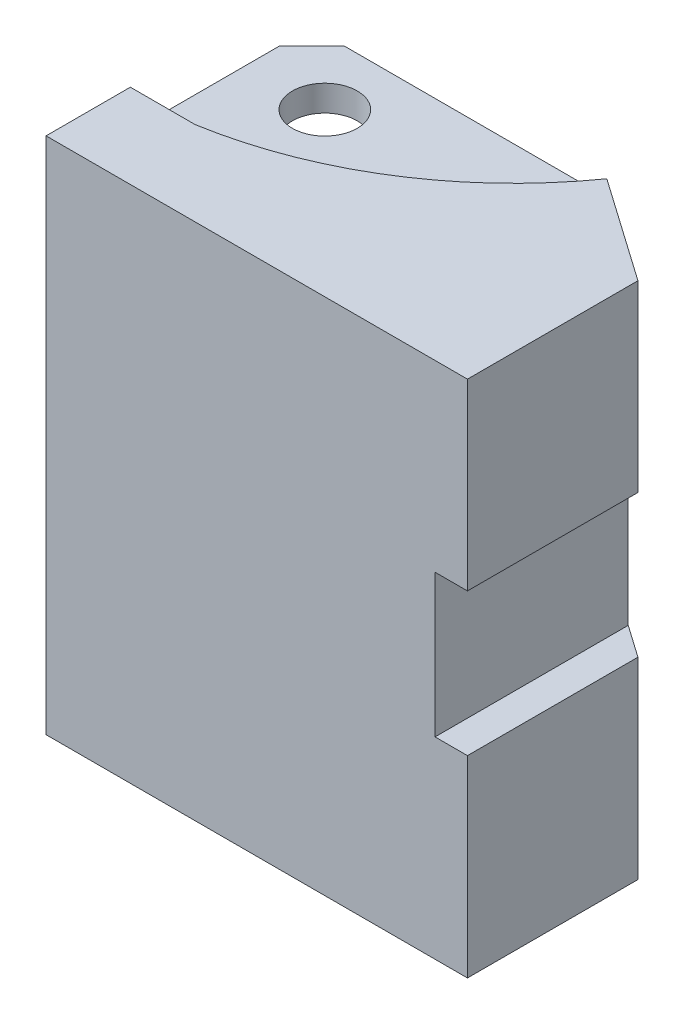
ISO-10303-21;
HEADER;
FILE_DESCRIPTION(('STEP AP214'),'2;1');
FILE_NAME('part.step','',(''),(''),'','','');
FILE_SCHEMA(('AUTOMOTIVE_DESIGN { 1 0 10303 214 1 1 1 1 }'));
ENDSEC;
DATA;
#1=APPLICATION_CONTEXT('core data for automotive mechanical design processes');
#2=APPLICATION_PROTOCOL_DEFINITION('international standard','automotive_design',2000,#1);
#3=PRODUCT_CONTEXT('',#1,'mechanical');
#4=PRODUCT('Part','Part','',(#3));
#5=PRODUCT_RELATED_PRODUCT_CATEGORY('part','',(#4));
#6=PRODUCT_DEFINITION_FORMATION('','',#4);
#7=PRODUCT_DEFINITION_CONTEXT('part definition',#1,'design');
#8=PRODUCT_DEFINITION('design','',#6,#7);
#9=PRODUCT_DEFINITION_SHAPE('','',#8);
#10=(LENGTH_UNIT() NAMED_UNIT(*) SI_UNIT(.MILLI.,.METRE.));
#11=(NAMED_UNIT(*) PLANE_ANGLE_UNIT() SI_UNIT($,.RADIAN.));
#12=(NAMED_UNIT(*) SI_UNIT($,.STERADIAN.) SOLID_ANGLE_UNIT());
#13=UNCERTAINTY_MEASURE_WITH_UNIT(LENGTH_MEASURE(1.E-05),#10,'distance_accuracy_value','');
#14=(GEOMETRIC_REPRESENTATION_CONTEXT(3) GLOBAL_UNCERTAINTY_ASSIGNED_CONTEXT((#13)) GLOBAL_UNIT_ASSIGNED_CONTEXT((#10,
#11,#12)) REPRESENTATION_CONTEXT('',''));
#15=CARTESIAN_POINT('',(0.,0.,0.));
#16=DIRECTION('',(0.,0.,1.));
#17=DIRECTION('',(1.,0.,0.));
#18=AXIS2_PLACEMENT_3D('',#15,#16,#17);
#19=CARTESIAN_POINT('',(-27.5,40.,-20.5));
#20=DIRECTION('',(0.,0.,1.));
#21=DIRECTION('',(1.,0.,0.));
#22=AXIS2_PLACEMENT_3D('',#19,#20,#21);
#23=PLANE('',#22);
#24=DIRECTION('',(-1.,0.,0.));
#25=VECTOR('',#24,1.);
#26=CARTESIAN_POINT('',(11.5,-30.,-20.5));
#27=LINE('',#26,#25);
#28=CARTESIAN_POINT('',(11.5,-30.,-20.5));
#29=VERTEX_POINT('',#28);
#30=CARTESIAN_POINT('',(-27.5,-30.,-20.5));
#31=VERTEX_POINT('',#30);
#32=EDGE_CURVE('E175',#29,#31,#27,.T.);
#33=ORIENTED_EDGE('',*,*,#32,.F.);
#34=DIRECTION('',(0.,-1.,0.));
#35=VECTOR('',#34,1.);
#36=CARTESIAN_POINT('',(11.5,40.,-20.5));
#37=LINE('',#36,#35);
#38=CARTESIAN_POINT('',(11.5,-40.,-20.5));
#39=VERTEX_POINT('',#38);
#40=EDGE_CURVE('E203',#29,#39,#37,.T.);
#41=ORIENTED_EDGE('',*,*,#40,.T.);
#42=DIRECTION('',(-1.,0.,0.));
#43=VECTOR('',#42,1.);
#44=CARTESIAN_POINT('',(-27.5,-40.,-20.5));
#45=LINE('',#44,#43);
#46=CARTESIAN_POINT('',(-27.5,-40.,-20.5));
#47=VERTEX_POINT('',#46);
#48=EDGE_CURVE('E194',#39,#47,#45,.T.);
#49=ORIENTED_EDGE('',*,*,#48,.T.);
#50=DIRECTION('',(0.,-1.,0.));
#51=VECTOR('',#50,1.);
#52=CARTESIAN_POINT('',(-27.5,40.,-20.5));
#53=LINE('',#52,#51);
#54=EDGE_CURVE('E189',#31,#47,#53,.T.);
#55=ORIENTED_EDGE('',*,*,#54,.F.);
#56=EDGE_LOOP('',(#33,#41,#49,#55));
#57=FACE_BOUND('',#56,.T.);
#58=ADVANCED_FACE('F39',(#57),#23,.F.);
#59=CARTESIAN_POINT('',(-32.5,40.,-15.5));
#60=DIRECTION('',(0.707106781186546,0.,0.707106781186549));
#61=DIRECTION('',(0.707106781186549,0.,-0.707106781186546));
#62=AXIS2_PLACEMENT_3D('',#59,#60,#61);
#63=PLANE('',#62);
#64=DIRECTION('',(-0.707106781186549,0.,0.707106781186546));
#65=VECTOR('',#64,1.);
#66=CARTESIAN_POINT('',(-27.5,-30.,-20.5));
#67=LINE('',#66,#65);
#68=CARTESIAN_POINT('',(-32.5,-30.,-15.5));
#69=VERTEX_POINT('',#68);
#70=EDGE_CURVE('E176',#31,#69,#67,.T.);
#71=ORIENTED_EDGE('',*,*,#70,.F.);
#72=ORIENTED_EDGE('',*,*,#54,.T.);
#73=DIRECTION('',(-0.707106781186549,0.,0.707106781186546));
#74=VECTOR('',#73,1.);
#75=CARTESIAN_POINT('',(-32.5,-40.,-15.5));
#76=LINE('',#75,#74);
#77=CARTESIAN_POINT('',(-32.5,-40.,-15.5));
#78=VERTEX_POINT('',#77);
#79=EDGE_CURVE('E261',#47,#78,#76,.T.);
#80=ORIENTED_EDGE('',*,*,#79,.T.);
#81=DIRECTION('',(0.,-1.,0.));
#82=VECTOR('',#81,1.);
#83=CARTESIAN_POINT('',(-32.5,40.,-15.5));
#84=LINE('',#83,#82);
#85=EDGE_CURVE('E191',#69,#78,#84,.T.);
#86=ORIENTED_EDGE('',*,*,#85,.F.);
#87=EDGE_LOOP('',(#71,#72,#80,#86));
#88=FACE_BOUND('',#87,.T.);
#89=ADVANCED_FACE('F190',(#88),#63,.F.);
#90=CARTESIAN_POINT('',(11.5,34.,-20.5));
#91=VERTEX_POINT('',#90);
#92=CARTESIAN_POINT('',(11.5,30.,-20.5));
#93=VERTEX_POINT('',#92);
#94=EDGE_CURVE('E206',#91,#93,#37,.T.);
#95=ORIENTED_EDGE('',*,*,#94,.T.);
#96=DIRECTION('',(-1.,0.,0.));
#97=VECTOR('',#96,1.);
#98=CARTESIAN_POINT('',(11.5,30.,-20.5));
#99=LINE('',#98,#97);
#100=CARTESIAN_POINT('',(-27.5,30.,-20.5));
#101=VERTEX_POINT('',#100);
#102=EDGE_CURVE('E341',#93,#101,#99,.T.);
#103=ORIENTED_EDGE('',*,*,#102,.T.);
#104=CARTESIAN_POINT('',(-27.5,34.,-20.5));
#105=VERTEX_POINT('',#104);
#106=EDGE_CURVE('E197',#105,#101,#53,.T.);
#107=ORIENTED_EDGE('',*,*,#106,.F.);
#108=DIRECTION('',(-1.,0.,0.));
#109=VECTOR('',#108,1.);
#110=CARTESIAN_POINT('',(11.5,34.,-20.5));
#111=LINE('',#110,#109);
#112=EDGE_CURVE('E318',#91,#105,#111,.T.);
#113=ORIENTED_EDGE('',*,*,#112,.F.);
#114=EDGE_LOOP('',(#95,#103,#107,#113));
#115=FACE_BOUND('',#114,.T.);
#116=ADVANCED_FACE('F377',(#115),#23,.F.);
#117=ORIENTED_EDGE('',*,*,#106,.T.);
#118=DIRECTION('',(-0.707106781186549,0.,0.707106781186546));
#119=VECTOR('',#118,1.);
#120=CARTESIAN_POINT('',(-27.5,30.,-20.5));
#121=LINE('',#120,#119);
#122=CARTESIAN_POINT('',(-32.5,30.,-15.5));
#123=VERTEX_POINT('',#122);
#124=EDGE_CURVE('E338',#101,#123,#121,.T.);
#125=ORIENTED_EDGE('',*,*,#124,.T.);
#126=CARTESIAN_POINT('',(-32.5,34.,-15.5));
#127=VERTEX_POINT('',#126);
#128=EDGE_CURVE('E196',#127,#123,#84,.T.);
#129=ORIENTED_EDGE('',*,*,#128,.F.);
#130=DIRECTION('',(-0.707106781186549,0.,0.707106781186546));
#131=VECTOR('',#130,1.);
#132=CARTESIAN_POINT('',(-27.5,34.,-20.5));
#133=LINE('',#132,#131);
#134=EDGE_CURVE('E316',#105,#127,#133,.T.);
#135=ORIENTED_EDGE('',*,*,#134,.F.);
#136=EDGE_LOOP('',(#117,#125,#129,#135));
#137=FACE_BOUND('',#136,.T.);
#138=ADVANCED_FACE('F384',(#137),#63,.F.);
#139=CARTESIAN_POINT('',(-32.5,40.,-15.5));
#140=DIRECTION('',(1.,0.,0.));
#141=DIRECTION('',(0.,0.,-1.));
#142=AXIS2_PLACEMENT_3D('',#139,#140,#141);
#143=PLANE('',#142);
#144=ORIENTED_EDGE('',*,*,#128,.T.);
#145=DIRECTION('',(0.,0.,1.));
#146=VECTOR('',#145,1.);
#147=CARTESIAN_POINT('',(-32.5,30.,-15.5));
#148=LINE('',#147,#146);
#149=CARTESIAN_POINT('',(-32.5,30.,7.5));
#150=VERTEX_POINT('',#149);
#151=EDGE_CURVE('E333',#123,#150,#148,.T.);
#152=ORIENTED_EDGE('',*,*,#151,.T.);
#153=DIRECTION('',(0.,1.,0.));
#154=VECTOR('',#153,1.);
#155=CARTESIAN_POINT('',(-32.5,-30.,7.5));
#156=LINE('',#155,#154);
#157=CARTESIAN_POINT('',(-32.5,-30.,7.5));
#158=VERTEX_POINT('',#157);
#159=EDGE_CURVE('E322',#158,#150,#156,.T.);
#160=ORIENTED_EDGE('',*,*,#159,.F.);
#161=DIRECTION('',(0.,0.,1.));
#162=VECTOR('',#161,1.);
#163=CARTESIAN_POINT('',(-32.5,-30.,-15.5));
#164=LINE('',#163,#162);
#165=EDGE_CURVE('E195',#69,#158,#164,.T.);
#166=ORIENTED_EDGE('',*,*,#165,.F.);
#167=ORIENTED_EDGE('',*,*,#85,.T.);
#168=DIRECTION('',(0.,0.,1.));
#169=VECTOR('',#168,1.);
#170=CARTESIAN_POINT('',(-32.5,-40.,-15.5));
#171=LINE('',#170,#169);
#172=CARTESIAN_POINT('',(-32.5,-40.,20.5));
#173=VERTEX_POINT('',#172);
#174=EDGE_CURVE('E263',#78,#173,#171,.T.);
#175=ORIENTED_EDGE('',*,*,#174,.T.);
#176=DIRECTION('',(0.,-1.,0.));
#177=VECTOR('',#176,1.);
#178=CARTESIAN_POINT('',(-32.5,40.,20.5));
#179=LINE('',#178,#177);
#180=CARTESIAN_POINT('',(-32.5,40.,20.5));
#181=VERTEX_POINT('',#180);
#182=EDGE_CURVE('E267',#181,#173,#179,.T.);
#183=ORIENTED_EDGE('',*,*,#182,.F.);
#184=DIRECTION('',(0.,0.,1.));
#185=VECTOR('',#184,1.);
#186=CARTESIAN_POINT('',(-32.5,40.,-15.5));
#187=LINE('',#186,#185);
#188=CARTESIAN_POINT('',(-32.5,40.,7.5));
#189=VERTEX_POINT('',#188);
#190=EDGE_CURVE('E251',#189,#181,#187,.T.);
#191=ORIENTED_EDGE('',*,*,#190,.F.);
#192=DIRECTION('',(0.,1.,0.));
#193=VECTOR('',#192,1.);
#194=CARTESIAN_POINT('',(-32.5,34.,7.5));
#195=LINE('',#194,#193);
#196=CARTESIAN_POINT('',(-32.5,34.,7.5));
#197=VERTEX_POINT('',#196);
#198=EDGE_CURVE('E63',#197,#189,#195,.T.);
#199=ORIENTED_EDGE('',*,*,#198,.F.);
#200=DIRECTION('',(0.,0.,1.));
#201=VECTOR('',#200,1.);
#202=CARTESIAN_POINT('',(-32.5,34.,-15.5));
#203=LINE('',#202,#201);
#204=EDGE_CURVE('E314',#127,#197,#203,.T.);
#205=ORIENTED_EDGE('',*,*,#204,.F.);
#206=EDGE_LOOP('',(#144,#152,#160,#166,#167,#175,#183,#191,#199,#205));
#207=FACE_BOUND('',#206,.T.);
#208=ADVANCED_FACE('F277',(#207),#143,.F.);
#209=CARTESIAN_POINT('',(32.5,40.,-5.79564169759613));
#210=DIRECTION('',(-1.,0.,0.));
#211=DIRECTION('',(0.,0.,1.));
#212=AXIS2_PLACEMENT_3D('',#209,#210,#211);
#213=PLANE('',#212);
#214=DIRECTION('',(0.,0.,-1.));
#215=VECTOR('',#214,1.);
#216=CARTESIAN_POINT('',(32.5,-10.2924598410793,20.5));
#217=LINE('',#216,#215);
#218=CARTESIAN_POINT('',(32.5,-10.2924598410793,20.5));
#219=VERTEX_POINT('',#218);
#220=CARTESIAN_POINT('',(32.5,-10.2924598410793,-5.79564169759612));
#221=VERTEX_POINT('',#220);
#222=EDGE_CURVE('E222',#219,#221,#217,.T.);
#223=ORIENTED_EDGE('',*,*,#222,.F.);
#224=DIRECTION('',(0.,-1.,0.));
#225=VECTOR('',#224,1.);
#226=CARTESIAN_POINT('',(32.5,40.,20.5));
#227=LINE('',#226,#225);
#228=CARTESIAN_POINT('',(32.5,-40.,20.5));
#229=VERTEX_POINT('',#228);
#230=EDGE_CURVE('E258',#219,#229,#227,.T.);
#231=ORIENTED_EDGE('',*,*,#230,.T.);
#232=DIRECTION('',(0.,0.,-1.));
#233=VECTOR('',#232,1.);
#234=CARTESIAN_POINT('',(32.5,-40.,-5.79564169759613));
#235=LINE('',#234,#233);
#236=CARTESIAN_POINT('',(32.5,-40.,-5.79564169759613));
#237=VERTEX_POINT('',#236);
#238=EDGE_CURVE('E237',#229,#237,#235,.T.);
#239=ORIENTED_EDGE('',*,*,#238,.T.);
#240=DIRECTION('',(0.,-1.,0.));
#241=VECTOR('',#240,1.);
#242=CARTESIAN_POINT('',(32.5,40.,-5.79564169759613));
#243=LINE('',#242,#241);
#244=EDGE_CURVE('E207',#221,#237,#243,.T.);
#245=ORIENTED_EDGE('',*,*,#244,.F.);
#246=EDGE_LOOP('',(#223,#231,#239,#245));
#247=FACE_BOUND('',#246,.T.);
#248=ADVANCED_FACE('F287',(#247),#213,.F.);
#249=CARTESIAN_POINT('',(11.5,40.,-20.5));
#250=DIRECTION('',(-0.573576436351045,0.,0.819152044288992));
#251=DIRECTION('',(0.819152044288992,0.,0.573576436351045));
#252=AXIS2_PLACEMENT_3D('',#249,#250,#251);
#253=PLANE('',#252);
#254=DIRECTION('',(0.,1.,0.));
#255=VECTOR('',#254,1.);
#256=CARTESIAN_POINT('',(16.4833271456414,-30.,-17.0106367672569));
#257=LINE('',#256,#255);
#258=CARTESIAN_POINT('',(16.4833271456414,-30.,-17.0106367672569));
#259=VERTEX_POINT('',#258);
#260=CARTESIAN_POINT('',(16.4833271456414,30.,-17.0106367672569));
#261=VERTEX_POINT('',#260);
#262=EDGE_CURVE('E313',#259,#261,#257,.T.);
#263=ORIENTED_EDGE('',*,*,#262,.T.);
#264=DIRECTION('',(-0.819152044288993,0.,-0.573576436351044));
#265=VECTOR('',#264,1.);
#266=CARTESIAN_POINT('',(16.4833271456413,30.,-17.0106367672569));
#267=LINE('',#266,#265);
#268=EDGE_CURVE('E54',#261,#93,#267,.T.);
#269=ORIENTED_EDGE('',*,*,#268,.T.);
#270=ORIENTED_EDGE('',*,*,#94,.F.);
#271=DIRECTION('',(-0.819152044288993,0.,-0.573576436351044));
#272=VECTOR('',#271,1.);
#273=CARTESIAN_POINT('',(16.4833271456413,34.,-17.0106367672569));
#274=LINE('',#273,#272);
#275=CARTESIAN_POINT('',(16.4833271456413,34.,-17.0106367672569));
#276=VERTEX_POINT('',#275);
#277=EDGE_CURVE('E319',#276,#91,#274,.T.);
#278=ORIENTED_EDGE('',*,*,#277,.F.);
#279=DIRECTION('',(0.,1.,0.));
#280=VECTOR('',#279,1.);
#281=CARTESIAN_POINT('',(16.4833271456413,34.,-17.0106367672569));
#282=LINE('',#281,#280);
#283=CARTESIAN_POINT('',(16.4833271456413,40.,-17.0106367672569));
#284=VERTEX_POINT('',#283);
#285=EDGE_CURVE('E296',#276,#284,#282,.T.);
#286=ORIENTED_EDGE('',*,*,#285,.T.);
#287=DIRECTION('',(-0.819152044288992,0.,-0.573576436351045));
#288=VECTOR('',#287,1.);
#289=CARTESIAN_POINT('',(11.5,40.,-20.5));
#290=LINE('',#289,#288);
#291=CARTESIAN_POINT('',(32.5,40.,-5.79564169759613));
#292=VERTEX_POINT('',#291);
#293=EDGE_CURVE('E248',#292,#284,#290,.T.);
#294=ORIENTED_EDGE('',*,*,#293,.F.);
#295=CARTESIAN_POINT('',(32.5,11.7075401589207,-5.79564169759612));
#296=VERTEX_POINT('',#295);
#297=EDGE_CURVE('E209',#292,#296,#243,.T.);
#298=ORIENTED_EDGE('',*,*,#297,.T.);
#299=DIRECTION('',(0.819152044288992,0.,0.573576436351045));
#300=VECTOR('',#299,1.);
#301=CARTESIAN_POINT('',(11.5,11.7075401589207,-20.5));
#302=LINE('',#301,#300);
#303=CARTESIAN_POINT('',(27.5,11.7075401589207,-9.29667938864467));
#304=VERTEX_POINT('',#303);
#305=EDGE_CURVE('E11',#304,#296,#302,.T.);
#306=ORIENTED_EDGE('',*,*,#305,.F.);
#307=DIRECTION('',(0.,1.,0.));
#308=VECTOR('',#307,1.);
#309=CARTESIAN_POINT('',(27.5,40.,-9.29667938864467));
#310=LINE('',#309,#308);
#311=CARTESIAN_POINT('',(27.5,-10.2924598410793,-9.29667938864466));
#312=VERTEX_POINT('',#311);
#313=EDGE_CURVE('E230',#312,#304,#310,.T.);
#314=ORIENTED_EDGE('',*,*,#313,.F.);
#315=DIRECTION('',(-0.819152044288992,0.,-0.573576436351045));
#316=VECTOR('',#315,1.);
#317=CARTESIAN_POINT('',(11.5,-10.2924598410793,-20.5));
#318=LINE('',#317,#316);
#319=EDGE_CURVE('E48',#221,#312,#318,.T.);
#320=ORIENTED_EDGE('',*,*,#319,.F.);
#321=ORIENTED_EDGE('',*,*,#244,.T.);
#322=DIRECTION('',(-0.819152044288992,0.,-0.573576436351045));
#323=VECTOR('',#322,1.);
#324=CARTESIAN_POINT('',(11.5,-40.,-20.5));
#325=LINE('',#324,#323);
#326=EDGE_CURVE('E238',#237,#39,#325,.T.);
#327=ORIENTED_EDGE('',*,*,#326,.T.);
#328=ORIENTED_EDGE('',*,*,#40,.F.);
#329=DIRECTION('',(-0.819152044288993,0.,-0.573576436351044));
#330=VECTOR('',#329,1.);
#331=CARTESIAN_POINT('',(16.4833271456413,-30.,-17.0106367672569));
#332=LINE('',#331,#330);
#333=EDGE_CURVE('E179',#259,#29,#332,.T.);
#334=ORIENTED_EDGE('',*,*,#333,.F.);
#335=EDGE_LOOP('',(#263,#269,#270,#278,#286,#294,#298,#306,#314,#320,#321,#327,#328,#334));
#336=FACE_BOUND('',#335,.T.);
#337=ADVANCED_FACE('F234',(#336),#253,.F.);
#338=CARTESIAN_POINT('',(-32.5,40.,20.5));
#339=DIRECTION('',(0.,0.,-1.));
#340=DIRECTION('',(-1.,0.,0.));
#341=AXIS2_PLACEMENT_3D('',#338,#339,#340);
#342=PLANE('',#341);
#343=DIRECTION('',(-1.,0.,0.));
#344=VECTOR('',#343,1.);
#345=CARTESIAN_POINT('',(27.5,11.7075401589207,20.5));
#346=LINE('',#345,#344);
#347=CARTESIAN_POINT('',(32.5,11.7075401589207,20.5));
#348=VERTEX_POINT('',#347);
#349=CARTESIAN_POINT('',(27.5,11.7075401589207,20.5));
#350=VERTEX_POINT('',#349);
#351=EDGE_CURVE('E293',#348,#350,#346,.T.);
#352=ORIENTED_EDGE('',*,*,#351,.F.);
#353=CARTESIAN_POINT('',(32.5,40.,20.5));
#354=VERTEX_POINT('',#353);
#355=EDGE_CURVE('E270',#354,#348,#227,.T.);
#356=ORIENTED_EDGE('',*,*,#355,.F.);
#357=DIRECTION('',(1.,0.,0.));
#358=VECTOR('',#357,1.);
#359=CARTESIAN_POINT('',(-32.5,40.,20.5));
#360=LINE('',#359,#358);
#361=EDGE_CURVE('E254',#181,#354,#360,.T.);
#362=ORIENTED_EDGE('',*,*,#361,.F.);
#363=ORIENTED_EDGE('',*,*,#182,.T.);
#364=DIRECTION('',(1.,0.,0.));
#365=VECTOR('',#364,1.);
#366=CARTESIAN_POINT('',(-32.5,-40.,20.5));
#367=LINE('',#366,#365);
#368=EDGE_CURVE('E249',#173,#229,#367,.T.);
#369=ORIENTED_EDGE('',*,*,#368,.T.);
#370=ORIENTED_EDGE('',*,*,#230,.F.);
#371=DIRECTION('',(1.,0.,0.));
#372=VECTOR('',#371,1.);
#373=CARTESIAN_POINT('',(27.5,-10.2924598410793,20.5));
#374=LINE('',#373,#372);
#375=CARTESIAN_POINT('',(27.5,-10.2924598410793,20.5));
#376=VERTEX_POINT('',#375);
#377=EDGE_CURVE('E286',#376,#219,#374,.T.);
#378=ORIENTED_EDGE('',*,*,#377,.F.);
#379=DIRECTION('',(0.,-1.,0.));
#380=VECTOR('',#379,1.);
#381=CARTESIAN_POINT('',(27.5,-10.2924598410793,20.5));
#382=LINE('',#381,#380);
#383=EDGE_CURVE('E226',#350,#376,#382,.T.);
#384=ORIENTED_EDGE('',*,*,#383,.F.);
#385=EDGE_LOOP('',(#352,#356,#362,#363,#369,#370,#378,#384));
#386=FACE_BOUND('',#385,.T.);
#387=ADVANCED_FACE('F281',(#386),#342,.F.);
#388=ORIENTED_EDGE('',*,*,#355,.T.);
#389=DIRECTION('',(0.,0.,-1.));
#390=VECTOR('',#389,1.);
#391=CARTESIAN_POINT('',(32.5,11.7075401589207,20.5));
#392=LINE('',#391,#390);
#393=EDGE_CURVE('E240',#348,#296,#392,.T.);
#394=ORIENTED_EDGE('',*,*,#393,.T.);
#395=ORIENTED_EDGE('',*,*,#297,.F.);
#396=DIRECTION('',(0.,0.,-1.));
#397=VECTOR('',#396,1.);
#398=CARTESIAN_POINT('',(32.5,40.,-5.79564169759613));
#399=LINE('',#398,#397);
#400=EDGE_CURVE('E246',#354,#292,#399,.T.);
#401=ORIENTED_EDGE('',*,*,#400,.F.);
#402=EDGE_LOOP('',(#388,#394,#395,#401));
#403=FACE_BOUND('',#402,.T.);
#404=ADVANCED_FACE('F41',(#403),#213,.F.);
#405=CARTESIAN_POINT('',(0.,40.,0.));
#406=DIRECTION('',(0.,1.,0.));
#407=DIRECTION('',(0.,0.,1.));
#408=AXIS2_PLACEMENT_3D('',#405,#406,#407);
#409=PLANE('',#408);
#410=CARTESIAN_POINT('',(-32.5,40.,-51.6607978309962));
#411=DIRECTION('',(0.,1.,0.));
#412=DIRECTION('',(0.,0.,1.));
#413=AXIS2_PLACEMENT_3D('',#410,#411,#412);
#414=CIRCLE('',#413,60.);
#415=CARTESIAN_POINT('',(-22.5,40.,7.5));
#416=VERTEX_POINT('',#415);
#417=EDGE_CURVE('E310',#416,#284,#414,.T.);
#418=ORIENTED_EDGE('',*,*,#417,.F.);
#419=DIRECTION('',(1.,0.,0.));
#420=VECTOR('',#419,1.);
#421=CARTESIAN_POINT('',(-32.5,40.,7.5));
#422=LINE('',#421,#420);
#423=EDGE_CURVE('E308',#189,#416,#422,.T.);
#424=ORIENTED_EDGE('',*,*,#423,.F.);
#425=ORIENTED_EDGE('',*,*,#190,.T.);
#426=ORIENTED_EDGE('',*,*,#361,.T.);
#427=ORIENTED_EDGE('',*,*,#400,.T.);
#428=ORIENTED_EDGE('',*,*,#293,.T.);
#429=EDGE_LOOP('',(#418,#424,#425,#426,#427,#428));
#430=FACE_BOUND('',#429,.T.);
#431=ADVANCED_FACE('F415',(#430),#409,.T.);
#432=CARTESIAN_POINT('',(0.,-40.,0.));
#433=DIRECTION('',(0.,1.,0.));
#434=DIRECTION('',(0.,0.,1.));
#435=AXIS2_PLACEMENT_3D('',#432,#433,#434);
#436=PLANE('',#435);
#437=CARTESIAN_POINT('',(-20.5,-40.,-10.5));
#438=DIRECTION('',(0.,1.,0.));
#439=DIRECTION('',(0.,0.,1.));
#440=AXIS2_PLACEMENT_3D('',#437,#438,#439);
#441=CIRCLE('',#440,5.);
#442=CARTESIAN_POINT('',(-20.5,-40.,-5.5));
#443=VERTEX_POINT('',#442);
#444=EDGE_CURVE('E343',#443,#443,#441,.T.);
#445=ORIENTED_EDGE('',*,*,#444,.T.);
#446=EDGE_LOOP('',(#445));
#447=FACE_BOUND('',#446,.T.);
#448=ORIENTED_EDGE('',*,*,#238,.F.);
#449=ORIENTED_EDGE('',*,*,#368,.F.);
#450=ORIENTED_EDGE('',*,*,#174,.F.);
#451=ORIENTED_EDGE('',*,*,#79,.F.);
#452=ORIENTED_EDGE('',*,*,#48,.F.);
#453=ORIENTED_EDGE('',*,*,#326,.F.);
#454=EDGE_LOOP('',(#448,#449,#450,#451,#452,#453));
#455=FACE_BOUND('',#454,.T.);
#456=ADVANCED_FACE('F282',(#447,#455),#436,.F.);
#457=CARTESIAN_POINT('',(27.5,11.7075401589207,20.5));
#458=DIRECTION('',(0.,-1.,0.));
#459=DIRECTION('',(0.,0.,-1.));
#460=AXIS2_PLACEMENT_3D('',#457,#458,#459);
#461=PLANE('',#460);
#462=ORIENTED_EDGE('',*,*,#305,.T.);
#463=ORIENTED_EDGE('',*,*,#393,.F.);
#464=ORIENTED_EDGE('',*,*,#351,.T.);
#465=DIRECTION('',(0.,0.,-1.));
#466=VECTOR('',#465,1.);
#467=CARTESIAN_POINT('',(27.5,11.7075401589207,20.5));
#468=LINE('',#467,#466);
#469=EDGE_CURVE('E231',#350,#304,#468,.T.);
#470=ORIENTED_EDGE('',*,*,#469,.T.);
#471=EDGE_LOOP('',(#462,#463,#464,#470));
#472=FACE_BOUND('',#471,.T.);
#473=ADVANCED_FACE('F294',(#472),#461,.T.);
#474=CARTESIAN_POINT('',(27.5,-10.2924598410793,20.5));
#475=DIRECTION('',(0.,1.,0.));
#476=DIRECTION('',(0.,0.,1.));
#477=AXIS2_PLACEMENT_3D('',#474,#475,#476);
#478=PLANE('',#477);
#479=ORIENTED_EDGE('',*,*,#319,.T.);
#480=DIRECTION('',(0.,0.,-1.));
#481=VECTOR('',#480,1.);
#482=CARTESIAN_POINT('',(27.5,-10.2924598410793,20.5));
#483=LINE('',#482,#481);
#484=EDGE_CURVE('E217',#376,#312,#483,.T.);
#485=ORIENTED_EDGE('',*,*,#484,.F.);
#486=ORIENTED_EDGE('',*,*,#377,.T.);
#487=ORIENTED_EDGE('',*,*,#222,.T.);
#488=EDGE_LOOP('',(#479,#485,#486,#487));
#489=FACE_BOUND('',#488,.T.);
#490=ADVANCED_FACE('F220',(#489),#478,.T.);
#491=CARTESIAN_POINT('',(27.5,-10.2924598410793,20.5));
#492=DIRECTION('',(1.,0.,0.));
#493=DIRECTION('',(0.,0.,-1.));
#494=AXIS2_PLACEMENT_3D('',#491,#492,#493);
#495=PLANE('',#494);
#496=ORIENTED_EDGE('',*,*,#313,.T.);
#497=ORIENTED_EDGE('',*,*,#469,.F.);
#498=ORIENTED_EDGE('',*,*,#383,.T.);
#499=ORIENTED_EDGE('',*,*,#484,.T.);
#500=EDGE_LOOP('',(#496,#497,#498,#499));
#501=FACE_BOUND('',#500,.T.);
#502=ADVANCED_FACE('F227',(#501),#495,.T.);
#503=CARTESIAN_POINT('',(-32.5,34.,-51.6607978309962));
#504=DIRECTION('',(0.,1.,0.));
#505=DIRECTION('',(0.,0.,1.));
#506=AXIS2_PLACEMENT_3D('',#503,#504,#505);
#507=CYLINDRICAL_SURFACE('',#506,60.);
#508=ORIENTED_EDGE('',*,*,#417,.T.);
#509=ORIENTED_EDGE('',*,*,#285,.F.);
#510=CARTESIAN_POINT('',(-32.5,34.,-51.6607978309962));
#511=DIRECTION('',(0.,1.,0.));
#512=DIRECTION('',(0.,0.,1.));
#513=AXIS2_PLACEMENT_3D('',#510,#511,#512);
#514=CIRCLE('',#513,60.);
#515=CARTESIAN_POINT('',(-22.5,34.,7.5));
#516=VERTEX_POINT('',#515);
#517=EDGE_CURVE('E306',#516,#276,#514,.T.);
#518=ORIENTED_EDGE('',*,*,#517,.F.);
#519=DIRECTION('',(0.,1.,0.));
#520=VECTOR('',#519,1.);
#521=CARTESIAN_POINT('',(-22.5,34.,7.5));
#522=LINE('',#521,#520);
#523=EDGE_CURVE('E300',#516,#416,#522,.T.);
#524=ORIENTED_EDGE('',*,*,#523,.T.);
#525=EDGE_LOOP('',(#508,#509,#518,#524));
#526=FACE_BOUND('',#525,.T.);
#527=ADVANCED_FACE('F409',(#526),#507,.F.);
#528=CARTESIAN_POINT('',(-32.5,34.,7.5));
#529=DIRECTION('',(0.,0.,1.));
#530=DIRECTION('',(1.,0.,0.));
#531=AXIS2_PLACEMENT_3D('',#528,#529,#530);
#532=PLANE('',#531);
#533=ORIENTED_EDGE('',*,*,#423,.T.);
#534=ORIENTED_EDGE('',*,*,#523,.F.);
#535=DIRECTION('',(1.,0.,0.));
#536=VECTOR('',#535,1.);
#537=CARTESIAN_POINT('',(-32.5,34.,7.5));
#538=LINE('',#537,#536);
#539=EDGE_CURVE('E302',#197,#516,#538,.T.);
#540=ORIENTED_EDGE('',*,*,#539,.F.);
#541=ORIENTED_EDGE('',*,*,#198,.T.);
#542=EDGE_LOOP('',(#533,#534,#540,#541));
#543=FACE_BOUND('',#542,.T.);
#544=ADVANCED_FACE('F444',(#543),#532,.F.);
#545=CARTESIAN_POINT('',(-32.5,34.,-51.6607978309962));
#546=DIRECTION('',(0.,1.,0.));
#547=DIRECTION('',(0.,0.,1.));
#548=AXIS2_PLACEMENT_3D('',#545,#546,#547);
#549=PLANE('',#548);
#550=CARTESIAN_POINT('',(-20.5,34.,-10.5));
#551=DIRECTION('',(0.,1.,0.));
#552=DIRECTION('',(0.,0.,1.));
#553=AXIS2_PLACEMENT_3D('',#550,#551,#552);
#554=CIRCLE('',#553,5.);
#555=CARTESIAN_POINT('',(-20.5,34.,-5.5));
#556=VERTEX_POINT('',#555);
#557=EDGE_CURVE('E360',#556,#556,#554,.T.);
#558=ORIENTED_EDGE('',*,*,#557,.F.);
#559=EDGE_LOOP('',(#558));
#560=FACE_BOUND('',#559,.T.);
#561=ORIENTED_EDGE('',*,*,#517,.T.);
#562=ORIENTED_EDGE('',*,*,#277,.T.);
#563=ORIENTED_EDGE('',*,*,#112,.T.);
#564=ORIENTED_EDGE('',*,*,#134,.T.);
#565=ORIENTED_EDGE('',*,*,#204,.T.);
#566=ORIENTED_EDGE('',*,*,#539,.T.);
#567=EDGE_LOOP('',(#561,#562,#563,#564,#565,#566));
#568=FACE_BOUND('',#567,.T.);
#569=ADVANCED_FACE('F407',(#560,#568),#549,.T.);
#570=CARTESIAN_POINT('',(-32.5,-30.,-51.6607978309962));
#571=DIRECTION('',(0.,1.,0.));
#572=DIRECTION('',(0.,0.,1.));
#573=AXIS2_PLACEMENT_3D('',#570,#571,#572);
#574=CYLINDRICAL_SURFACE('',#573,60.);
#575=CARTESIAN_POINT('',(-32.5,30.,-51.6607978309962));
#576=DIRECTION('',(0.,1.,0.));
#577=DIRECTION('',(0.,0.,1.));
#578=AXIS2_PLACEMENT_3D('',#575,#576,#577);
#579=CIRCLE('',#578,60.);
#580=CARTESIAN_POINT('',(-22.5,30.,7.5));
#581=VERTEX_POINT('',#580);
#582=EDGE_CURVE('E329',#581,#261,#579,.T.);
#583=ORIENTED_EDGE('',*,*,#582,.T.);
#584=ORIENTED_EDGE('',*,*,#262,.F.);
#585=CARTESIAN_POINT('',(-32.5,-30.,-51.6607978309962));
#586=DIRECTION('',(0.,1.,0.));
#587=DIRECTION('',(0.,0.,1.));
#588=AXIS2_PLACEMENT_3D('',#585,#586,#587);
#589=CIRCLE('',#588,60.);
#590=CARTESIAN_POINT('',(-22.5,-30.,7.5));
#591=VERTEX_POINT('',#590);
#592=EDGE_CURVE('E347',#591,#259,#589,.T.);
#593=ORIENTED_EDGE('',*,*,#592,.F.);
#594=DIRECTION('',(0.,1.,0.));
#595=VECTOR('',#594,1.);
#596=CARTESIAN_POINT('',(-22.5,-30.,7.5));
#597=LINE('',#596,#595);
#598=EDGE_CURVE('E326',#591,#581,#597,.T.);
#599=ORIENTED_EDGE('',*,*,#598,.T.);
#600=EDGE_LOOP('',(#583,#584,#593,#599));
#601=FACE_BOUND('',#600,.T.);
#602=ADVANCED_FACE('F397',(#601),#574,.F.);
#603=CARTESIAN_POINT('',(-32.5,-30.,7.5));
#604=DIRECTION('',(0.,0.,1.));
#605=DIRECTION('',(1.,0.,0.));
#606=AXIS2_PLACEMENT_3D('',#603,#604,#605);
#607=PLANE('',#606);
#608=DIRECTION('',(1.,0.,0.));
#609=VECTOR('',#608,1.);
#610=CARTESIAN_POINT('',(-32.5,30.,7.5));
#611=LINE('',#610,#609);
#612=EDGE_CURVE('E335',#150,#581,#611,.T.);
#613=ORIENTED_EDGE('',*,*,#612,.T.);
#614=ORIENTED_EDGE('',*,*,#598,.F.);
#615=DIRECTION('',(1.,0.,0.));
#616=VECTOR('',#615,1.);
#617=CARTESIAN_POINT('',(-32.5,-30.,7.5));
#618=LINE('',#617,#616);
#619=EDGE_CURVE('E346',#158,#591,#618,.T.);
#620=ORIENTED_EDGE('',*,*,#619,.F.);
#621=ORIENTED_EDGE('',*,*,#159,.T.);
#622=EDGE_LOOP('',(#613,#614,#620,#621));
#623=FACE_BOUND('',#622,.T.);
#624=ADVANCED_FACE('F399',(#623),#607,.F.);
#625=CARTESIAN_POINT('',(-32.5,-30.,-51.6607978309962));
#626=DIRECTION('',(0.,1.,0.));
#627=DIRECTION('',(0.,0.,1.));
#628=AXIS2_PLACEMENT_3D('',#625,#626,#627);
#629=PLANE('',#628);
#630=CARTESIAN_POINT('',(-20.5,-30.,-10.5));
#631=DIRECTION('',(0.,1.,0.));
#632=DIRECTION('',(0.,0.,1.));
#633=AXIS2_PLACEMENT_3D('',#630,#631,#632);
#634=CIRCLE('',#633,5.);
#635=CARTESIAN_POINT('',(-20.5,-30.,-5.5));
#636=VERTEX_POINT('',#635);
#637=EDGE_CURVE('E354',#636,#636,#634,.T.);
#638=ORIENTED_EDGE('',*,*,#637,.F.);
#639=EDGE_LOOP('',(#638));
#640=FACE_BOUND('',#639,.T.);
#641=ORIENTED_EDGE('',*,*,#32,.T.);
#642=ORIENTED_EDGE('',*,*,#70,.T.);
#643=ORIENTED_EDGE('',*,*,#165,.T.);
#644=ORIENTED_EDGE('',*,*,#619,.T.);
#645=ORIENTED_EDGE('',*,*,#592,.T.);
#646=ORIENTED_EDGE('',*,*,#333,.T.);
#647=EDGE_LOOP('',(#641,#642,#643,#644,#645,#646));
#648=FACE_BOUND('',#647,.T.);
#649=ADVANCED_FACE('F174',(#640,#648),#629,.T.);
#650=CARTESIAN_POINT('',(-32.5,30.,-51.6607978309962));
#651=DIRECTION('',(0.,1.,0.));
#652=DIRECTION('',(0.,0.,1.));
#653=AXIS2_PLACEMENT_3D('',#650,#651,#652);
#654=PLANE('',#653);
#655=CARTESIAN_POINT('',(-20.5,30.,-10.5));
#656=DIRECTION('',(0.,1.,0.));
#657=DIRECTION('',(0.,0.,1.));
#658=AXIS2_PLACEMENT_3D('',#655,#656,#657);
#659=CIRCLE('',#658,5.);
#660=CARTESIAN_POINT('',(-20.5,30.,-5.5));
#661=VERTEX_POINT('',#660);
#662=EDGE_CURVE('E43',#661,#661,#659,.T.);
#663=ORIENTED_EDGE('',*,*,#662,.T.);
#664=EDGE_LOOP('',(#663));
#665=FACE_BOUND('',#664,.T.);
#666=ORIENTED_EDGE('',*,*,#102,.F.);
#667=ORIENTED_EDGE('',*,*,#268,.F.);
#668=ORIENTED_EDGE('',*,*,#582,.F.);
#669=ORIENTED_EDGE('',*,*,#612,.F.);
#670=ORIENTED_EDGE('',*,*,#151,.F.);
#671=ORIENTED_EDGE('',*,*,#124,.F.);
#672=EDGE_LOOP('',(#666,#667,#668,#669,#670,#671));
#673=FACE_BOUND('',#672,.T.);
#674=ADVANCED_FACE('F365',(#665,#673),#654,.F.);
#675=CARTESIAN_POINT('',(-20.5,-76.,-10.5));
#676=DIRECTION('',(0.,1.,0.));
#677=DIRECTION('',(0.,0.,1.));
#678=AXIS2_PLACEMENT_3D('',#675,#676,#677);
#679=CYLINDRICAL_SURFACE('',#678,5.);
#680=ORIENTED_EDGE('',*,*,#557,.T.);
#681=EDGE_LOOP('',(#680));
#682=FACE_BOUND('',#681,.T.);
#683=ORIENTED_EDGE('',*,*,#662,.F.);
#684=EDGE_LOOP('',(#683));
#685=FACE_BOUND('',#684,.T.);
#686=ADVANCED_FACE('F368',(#682,#685),#679,.F.);
#687=ORIENTED_EDGE('',*,*,#637,.T.);
#688=EDGE_LOOP('',(#687));
#689=FACE_BOUND('',#688,.T.);
#690=ORIENTED_EDGE('',*,*,#444,.F.);
#691=EDGE_LOOP('',(#690));
#692=FACE_BOUND('',#691,.T.);
#693=ADVANCED_FACE('F366',(#689,#692),#679,.F.);
#694=CLOSED_SHELL('',(#58,#89,#116,#138,#208,#248,#337,#387,#404,#431,#456,#473,#490,#502,#527,
#544,#569,#602,#624,#649,#674,#686,#693));
#695=MANIFOLD_SOLID_BREP('B2',#694);
#696=ADVANCED_BREP_SHAPE_REPRESENTATION('',(#18,#695),#14);
#697=SHAPE_DEFINITION_REPRESENTATION(#9,#696);
ENDSEC;
END-ISO-10303-21;
